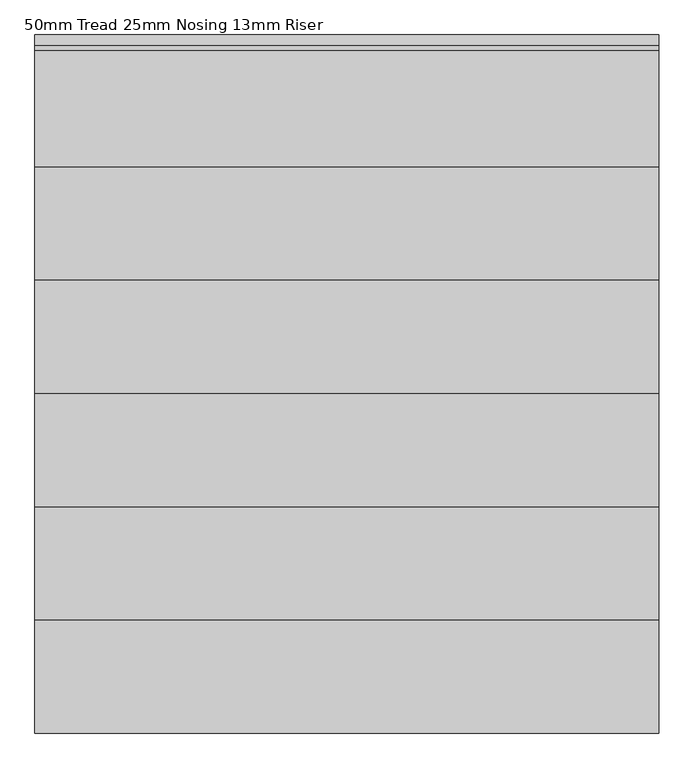
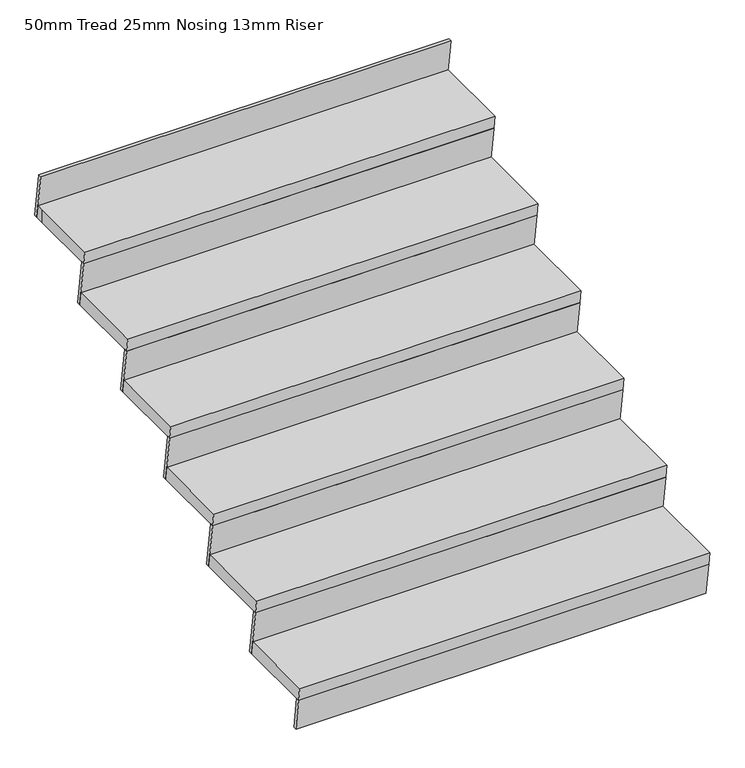
"""IFC4 building model written with IfcOpenShell, lengths in millimetres: stair flight geometry, 50mm Tread 25mm Nosing 13mm Riser."""

from ifc_helpers import new_model, si_unit, origin, place, context, project, spatial, faceted_brep, source, transform, mapped, element, save


def stair_flight_50mm_tread_25mm_nosing_13mm_riser_cb9873a3(model_context):
    return source(origin(), model_context, "Body", "Brep", [
        faceted_brep([(-866.6164824, 9042.1981148, 173.9130435), (-866.6164824, 9049.3856148, 123.9130435), (-2381.5205334, 9049.3856148, 123.9130435), (-2381.5205334, 9042.1981148, 173.9130435), (-2381.5205334, 8742.1981148, 173.9130435), (-866.6164824, 8742.1981148, 173.9130435), (-866.6164824, 8749.3856148, 123.9130435), (-2381.5205334, 8749.3856148, 123.9130435)], [[[0, 1, 2, 3]], [[3, 4, 5, 0]], [[2, 1, 6, 7]], [[4, 3, 2, 7]], [[0, 5, 6, 1]], [[5, 4, 7, 6]]]),
        faceted_brep([(-866.6164824, 8749.3856148, 123.9130435), (-866.6164824, 8767.1981148, 0.0), (-866.6164824, 8779.8266048, 0.0), (-866.6164824, 8762.0141048, 123.9130435), (-2381.5205334, 8749.3856148, 123.9130435), (-2381.5205334, 8762.0141048, 123.9130435), (-2381.5205334, 8779.8266048, 0.0), (-2381.5205334, 8767.1981148, 0.0)], [[[0, 1, 2, 3]], [[4, 5, 6, 7]], [[1, 0, 4, 7]], [[2, 1, 7, 6]], [[3, 2, 6, 5]], [[0, 3, 5, 4]]]),
        faceted_brep([(-866.6164824, 9024.3856148, 297.826087), (-866.6164824, 9049.3856148, 123.9130435), (-866.6164824, 9062.0141048, 123.9130435), (-866.6164824, 9037.0141048, 297.826087), (-2381.5205334, 9024.3856148, 297.826087), (-2381.5205334, 9037.0141048, 297.826087), (-2381.5205334, 9062.0141048, 123.9130435), (-2381.5205334, 9049.3856148, 123.9130435)], [[[0, 1, 2, 3]], [[4, 5, 6, 7]], [[1, 0, 4, 7]], [[2, 1, 7, 6]], [[3, 2, 6, 5]], [[0, 3, 5, 4]]]),
        faceted_brep([(-2381.5205334, 9317.1981148, 347.826087), (-2381.5205334, 9017.1981148, 347.826087), (-866.6164824, 9017.1981148, 347.826087), (-866.6164824, 9317.1981148, 347.826087), (-2381.5205334, 9324.3856148, 297.826087), (-866.6164824, 9324.3856148, 297.826087), (-866.6164824, 9024.3856148, 297.826087), (-2381.5205334, 9024.3856148, 297.826087)], [[[0, 1, 2, 3]], [[4, 5, 6, 7]], [[1, 0, 4, 7]], [[3, 2, 6, 5]], [[3, 5, 4, 0]], [[2, 1, 7, 6]]]),
        faceted_brep([(-866.6164824, 9299.3856148, 471.7391304), (-866.6164824, 9324.3856148, 297.826087), (-866.6164824, 9337.0141048, 297.826087), (-866.6164824, 9312.0141048, 471.7391304), (-2381.5205334, 9299.3856148, 471.7391304), (-2381.5205334, 9312.0141048, 471.7391304), (-2381.5205334, 9337.0141048, 297.826087), (-2381.5205334, 9324.3856148, 297.826087)], [[[0, 1, 2, 3]], [[4, 5, 6, 7]], [[1, 0, 4, 7]], [[2, 1, 7, 6]], [[3, 2, 6, 5]], [[0, 3, 5, 4]]]),
        faceted_brep([(-2381.5205334, 9592.1981148, 521.7391304), (-2381.5205334, 9292.1981148, 521.7391304), (-866.6164824, 9292.1981148, 521.7391304), (-866.6164824, 9592.1981148, 521.7391304), (-2381.5205334, 9599.3856148, 471.7391304), (-866.6164824, 9599.3856148, 471.7391304), (-866.6164824, 9299.3856148, 471.7391304), (-2381.5205334, 9299.3856148, 471.7391304)], [[[0, 1, 2, 3]], [[4, 5, 6, 7]], [[1, 0, 4, 7]], [[3, 2, 6, 5]], [[3, 5, 4, 0]], [[2, 1, 7, 6]]]),
        faceted_brep([(-866.6164824, 9574.3856148, 645.6521739), (-866.6164824, 9599.3856148, 471.7391304), (-866.6164824, 9612.0141048, 471.7391304), (-866.6164824, 9587.0141048, 645.6521739), (-2381.5205334, 9574.3856148, 645.6521739), (-2381.5205334, 9587.0141048, 645.6521739), (-2381.5205334, 9612.0141048, 471.7391304), (-2381.5205334, 9599.3856148, 471.7391304)], [[[0, 1, 2, 3]], [[4, 5, 6, 7]], [[1, 0, 4, 7]], [[2, 1, 7, 6]], [[3, 2, 6, 5]], [[0, 3, 5, 4]]]),
        faceted_brep([(-2381.5205334, 9867.1981148, 695.6521739), (-2381.5205334, 9567.1981148, 695.6521739), (-866.6164824, 9567.1981148, 695.6521739), (-866.6164824, 9867.1981148, 695.6521739), (-2381.5205334, 9874.3856148, 645.6521739), (-866.6164824, 9874.3856148, 645.6521739), (-866.6164824, 9574.3856148, 645.6521739), (-2381.5205334, 9574.3856148, 645.6521739)], [[[0, 1, 2, 3]], [[4, 5, 6, 7]], [[1, 0, 4, 7]], [[3, 2, 6, 5]], [[3, 5, 4, 0]], [[2, 1, 7, 6]]]),
        faceted_brep([(-866.6164824, 9849.3856148, 819.5652174), (-866.6164824, 9874.3856148, 645.6521739), (-866.6164824, 9887.0141048, 645.6521739), (-866.6164824, 9862.0141048, 819.5652174), (-2381.5205334, 9849.3856148, 819.5652174), (-2381.5205334, 9862.0141048, 819.5652174), (-2381.5205334, 9887.0141048, 645.6521739), (-2381.5205334, 9874.3856148, 645.6521739)], [[[0, 1, 2, 3]], [[4, 5, 6, 7]], [[1, 0, 4, 7]], [[2, 1, 7, 6]], [[3, 2, 6, 5]], [[0, 3, 5, 4]]]),
        faceted_brep([(-2381.5205334, 10142.1981148, 869.5652174), (-2381.5205334, 9842.1981148, 869.5652174), (-866.6164824, 9842.1981148, 869.5652174), (-866.6164824, 10142.1981148, 869.5652174), (-2381.5205334, 10149.3856148, 819.5652174), (-866.6164824, 10149.3856148, 819.5652174), (-866.6164824, 9849.3856148, 819.5652174), (-2381.5205334, 9849.3856148, 819.5652174)], [[[0, 1, 2, 3]], [[4, 5, 6, 7]], [[1, 0, 4, 7]], [[3, 2, 6, 5]], [[3, 5, 4, 0]], [[2, 1, 7, 6]]]),
        faceted_brep([(-866.6164824, 10399.3856148, 1167.3913043), (-866.6164824, 10424.3856148, 993.4782609), (-866.6164824, 10437.0141048, 993.4782609), (-866.6164824, 10412.0141048, 1167.3913043), (-2381.5205334, 10399.3856148, 1167.3913043), (-2381.5205334, 10412.0141048, 1167.3913043), (-2381.5205334, 10437.0141048, 993.4782609), (-2381.5205334, 10424.3856148, 993.4782609)], [[[0, 1, 2, 3]], [[4, 5, 6, 7]], [[1, 0, 4, 7]], [[2, 1, 7, 6]], [[3, 2, 6, 5]], [[0, 3, 5, 4]]]),
        faceted_brep([(-866.6164824, 10124.3856148, 993.4782609), (-866.6164824, 10149.3856148, 819.5652174), (-866.6164824, 10162.0141048, 819.5652174), (-866.6164824, 10137.0141048, 993.4782609), (-2381.5205334, 10124.3856148, 993.4782609), (-2381.5205334, 10137.0141048, 993.4782609), (-2381.5205334, 10162.0141048, 819.5652174), (-2381.5205334, 10149.3856148, 819.5652174)], [[[0, 1, 2, 3]], [[4, 5, 6, 7]], [[1, 0, 4, 7]], [[2, 1, 7, 6]], [[3, 2, 6, 5]], [[0, 3, 5, 4]]]),
        faceted_brep([(-2381.5205334, 10417.1981148, 1043.4782609), (-2381.5205334, 10392.1981148, 1043.4782609), (-2381.5205334, 10117.1981148, 1043.4782609), (-866.6164824, 10117.1981148, 1043.4782609), (-866.6164824, 10417.1981148, 1043.4782609), (-2381.5205334, 10424.3856148, 993.4782609), (-866.6164824, 10424.3856148, 993.4782609), (-866.6164824, 10124.3856148, 993.4782609), (-2381.5205334, 10124.3856148, 993.4782609), (-2381.5205334, 10392.1981148, 993.4782609)], [[[0, 1, 2, 3, 4]], [[5, 6, 7, 8, 9]], [[1, 0, 5, 9]], [[2, 1, 9, 8]], [[4, 3, 7, 6]], [[4, 6, 5, 0]], [[3, 2, 8, 7]]]),
    ])


if __name__ == "__main__":
    model = new_model("IFC4")
    model_context = context("Model", 3, world=origin())
    ifc_project = project(units=[si_unit("LENGTHUNIT", "METRE", prefix="MILLI")], contexts=[model_context])
    site = spatial("IfcSite", under=ifc_project)
    building = spatial("IfcBuilding", under=site)
    placement = place(None, origin())
    stair_flight_50mm_tread_25mm_nosing_13mm_riser_shape = stair_flight_50mm_tread_25mm_nosing_13mm_riser_cb9873a3(model_context)
    element("IfcStairFlight", 1, ObjectType="50mm Tread 25mm Nosing 13mm Riser", at=placement, inside=building, context=model_context, shape_type="MappedRepresentation", body=[
        mapped(stair_flight_50mm_tread_25mm_nosing_13mm_riser_shape, transform((0.0, 0.0, 0.0), x_axis=(1.0, 0.0, 0.0), y_axis=(0.0, 1.0, 0.0), z_axis=(0.0, 0.0, 1.0))),
    ])
    save(model, "model.ifc")
